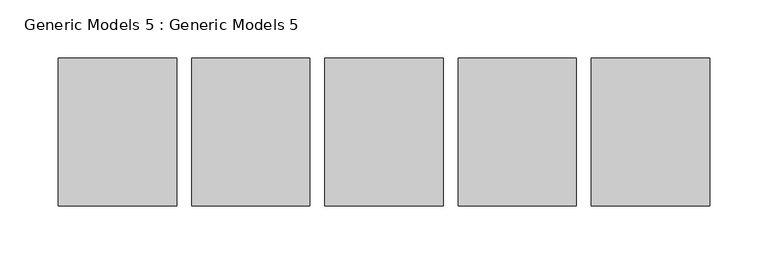
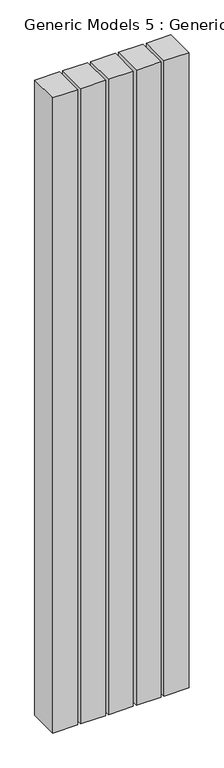
"""IFC4 building model written with IfcOpenShell, lengths in millimetres: proxy geometry, Generic Models 5 : Generic Models 5."""

from ifc_helpers import new_model, si_unit, frame, origin, place, context, project, spatial, polyline, outline, extrude, source, transform, mapped, element, save


def generic_models_5_generic_models_5_fe75d143(model_context):
    return source(origin(), model_context, "Body", "SweptSolid", [
        extrude(outline(polyline([(-3148.321199, -5879.7642512), (-3249.921199, -5879.7642512), (-3249.921199, -5752.7642512), (-3148.321199, -5752.7642512), (-3148.321199, -5879.7642512)])), frame((0.0, 0.0, 3352.8), z_axis=(0.0, 0.0, 1.0), x_axis=(1.0, 0.0, 0.0)), (0.0, 0.0, 1.0), 2750.7761011),
        extrude(outline(polyline([(-3034.021199, -5879.7642512), (-3135.621199, -5879.7642512), (-3135.621199, -5752.7642512), (-3034.021199, -5752.7642512), (-3034.021199, -5879.7642512)])), frame((0.0, 0.0, 3352.8), z_axis=(0.0, 0.0, 1.0), x_axis=(1.0, 0.0, 0.0)), (0.0, 0.0, 1.0), 2750.7761011),
        extrude(outline(polyline([(-2919.721199, -5879.7642512), (-3021.321199, -5879.7642512), (-3021.321199, -5752.7642512), (-2919.721199, -5752.7642512), (-2919.721199, -5879.7642512)])), frame((0.0, 0.0, 3352.8), z_axis=(0.0, 0.0, 1.0), x_axis=(1.0, 0.0, 0.0)), (0.0, 0.0, 1.0), 2750.7761011),
        extrude(outline(polyline([(-2805.421199, -5879.7642512), (-2907.021199, -5879.7642512), (-2907.021199, -5752.7642512), (-2805.421199, -5752.7642512), (-2805.421199, -5879.7642512)])), frame((0.0, 0.0, 3352.8), z_axis=(0.0, 0.0, 1.0), x_axis=(1.0, 0.0, 0.0)), (0.0, 0.0, 1.0), 2750.7761011),
        extrude(outline(polyline([(-2691.121199, -5879.7642512), (-2792.721199, -5879.7642512), (-2792.721199, -5752.7642512), (-2691.121199, -5752.7642512), (-2691.121199, -5879.7642512)])), frame((0.0, 0.0, 3352.8), z_axis=(0.0, 0.0, 1.0), x_axis=(1.0, 0.0, 0.0)), (0.0, 0.0, 1.0), 2750.7761011),
    ])


if __name__ == "__main__":
    model = new_model("IFC4")
    model_context = context("Model", 3, world=origin())
    ifc_project = project(units=[si_unit("LENGTHUNIT", "METRE", prefix="MILLI")], contexts=[model_context])
    site = spatial("IfcSite", under=ifc_project)
    building = spatial("IfcBuilding", under=site)
    placement = place(None, origin())
    generic_models_5_generic_models_5_shape = generic_models_5_generic_models_5_fe75d143(model_context)
    element("IfcBuildingElementProxy", 1, Name="Generic Models 5 : Generic Models 5", ObjectType="Generic Models 5 : Generic Models 5", at=placement, inside=building, context=model_context, shape_type="MappedRepresentation", body=[
        mapped(generic_models_5_generic_models_5_shape, transform((0.0, 0.0, 0.0), x_axis=(1.0, 0.0, 0.0), y_axis=(0.0, 1.0, 0.0), z_axis=(0.0, 0.0, 1.0))),
    ])
    save(model, "model.ifc")
